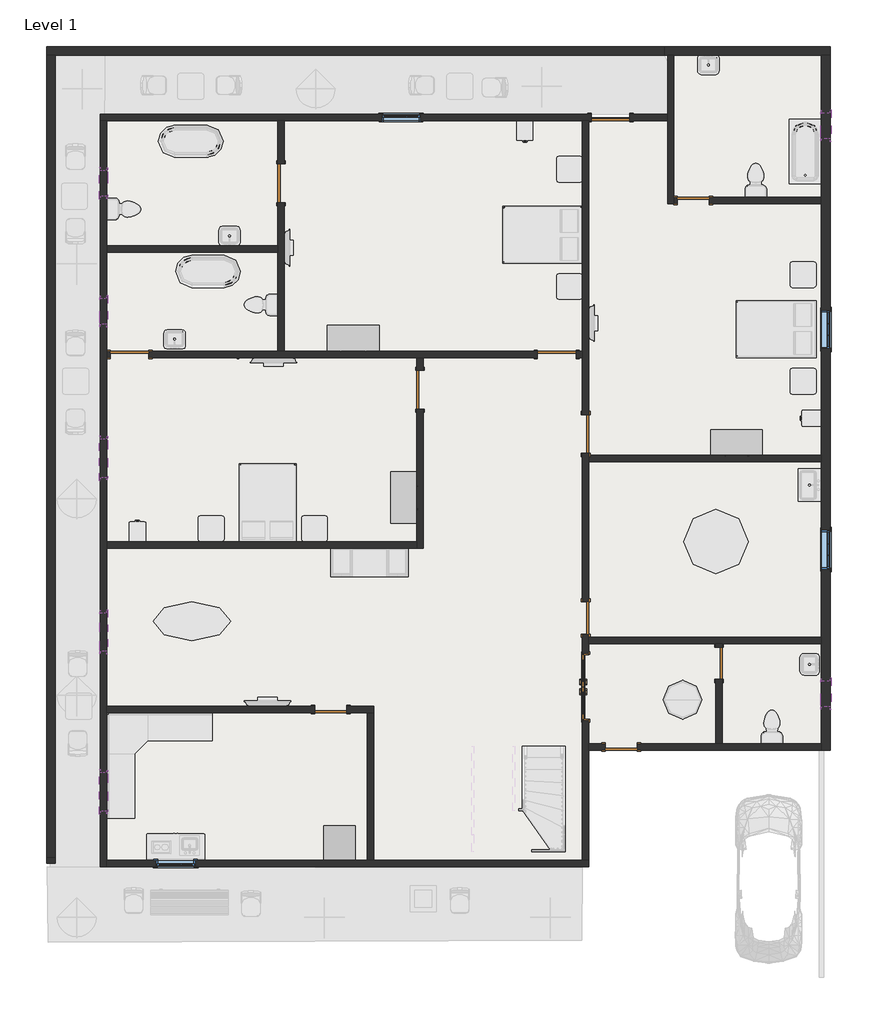
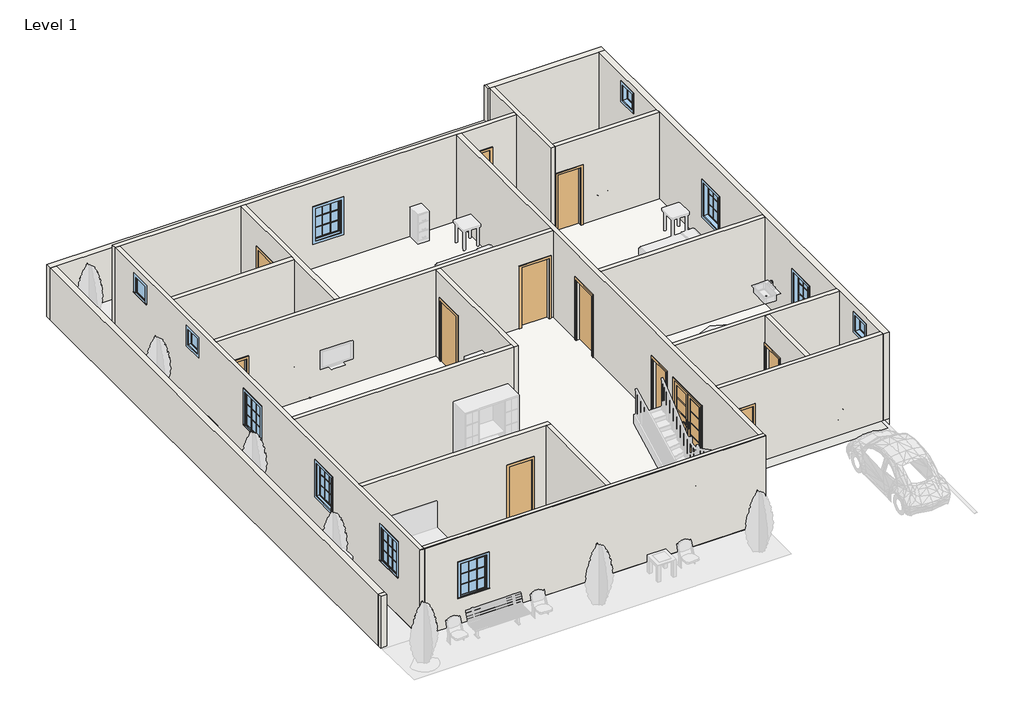
# One storey, part 1 of 3: 22 walls, 12 doors, 11 windows, 1 slab.
"""IFC4 building model written with IfcOpenShell, lengths in millimetres."""

from ifc_helpers import new_model, si_unit, frame, origin, origin_with_axes, place, context, project, spatial, polyline, outline, extrude, faceted_brep, transform, mapped, element, save
from components import door_94998e6c, door_255cab33, door_059fdd7e, door_16372e1c, door_686f89d2, window_5c190c7e, window_29c06734, window_e41d21a6, window_3d781103

model = new_model("IFC4")

# Units and contexts
model_context = context("Model", 3, world=origin())
ifc_project = project(units=[si_unit("LENGTHUNIT", "METRE", prefix="MILLI")], contexts=[model_context])

# Site, building, storey
site = spatial("IfcSite", under=ifc_project)
building = spatial("IfcBuilding", under=site)
storey = spatial("IfcBuildingStorey", under=building, Name="Level 1", Elevation=0.0)

# Doors
placement = place(None, origin())
door_shape = door_94998e6c(model_context)
element("IfcDoor", 1, ObjectType="Door-Exterior-Double-Full Glass-Wood_Clad : 60\" x 80\"", at=placement, inside=storey, context=model_context, shape_type="MappedRepresentation", body=[
    mapped(door_shape, transform((-2733.8668623, -1407.4089531, 0.0), x_axis=(0.0, 1.0, 0.0), y_axis=(-1.0, 0.0, 0.0), z_axis=(0.0, 0.0, 1.0))),
])
door_2_shape = door_255cab33(model_context)
element("IfcDoor", 2, ObjectType="Single-Flush : 30\" x 80\"", at=placement, inside=storey, context=model_context, shape_type="MappedRepresentation", body=[
    mapped(door_2_shape, transform((-190.6918623, 10073.3910469, 0.0), x_axis=(-1.0, 0.0, 0.0), y_axis=(0.0, -1.0, 0.0), z_axis=(0.0, 0.0, 1.0))),
])
element("IfcDoor", 3, ObjectType="Single-Flush : 30\" x 80\"", at=placement, inside=storey, context=model_context, shape_type="MappedRepresentation", body=[
    mapped(door_2_shape, transform((418.9081377, -848.6089531, 0.0), x_axis=(0.0, 1.0, 0.0), y_axis=(-1.0, 0.0, 0.0), z_axis=(0.0, 0.0, 1.0))),
])
element("IfcDoor", 4, ObjectType="Single-Flush : 30\" x 80\"", at=placement, inside=storey, context=model_context, shape_type="MappedRepresentation", body=[
    mapped(door_2_shape, transform((-8750.4918623, -1940.8089531, 0.0), x_axis=(1.0, 0.0, 0.0), y_axis=(0.0, 1.0, 0.0), z_axis=(0.0, 0.0, 1.0))),
])
door_3_shape = door_059fdd7e(model_context)
element("IfcDoor", 5, ObjectType="Single-Flush : 30\" x 80\"", at=placement, inside=storey, context=model_context, shape_type="MappedRepresentation", body=[
    mapped(door_3_shape, transform((-2730.6918623, 218.1910469, 0.0), x_axis=(0.0, -1.0, 0.0), y_axis=(1.0, 0.0, 0.0), z_axis=(0.0, 0.0, 1.0))),
])
element("IfcDoor", 6, ObjectType="Single-Flush : 30\" x 80\"", at=placement, inside=storey, context=model_context, shape_type="MappedRepresentation", body=[
    mapped(door_3_shape, transform((-1892.4918623, -2829.8089531, 0.0), x_axis=(-1.0, 0.0, 0.0), y_axis=(0.0, -1.0, 0.0), z_axis=(0.0, 0.0, 1.0))),
])
door_4_shape = door_16372e1c(model_context)
element("IfcDoor", 7, ObjectType="Single-Flush : 36\" x 84\"", at=placement, inside=storey, context=model_context, shape_type="MappedRepresentation", body=[
    mapped(door_4_shape, transform((-9918.8918623, 10479.7910469, 0.0), x_axis=(0.0, 1.0, 0.0), y_axis=(-1.0, 0.0, 0.0), z_axis=(0.0, 0.0, 1.0))),
])
element("IfcDoor", 8, ObjectType="Single-Flush : 36\" x 84\"", at=placement, inside=storey, context=model_context, shape_type="MappedRepresentation", body=[
    mapped(door_4_shape, transform((-6642.2918623, 5602.9910469, 0.0), x_axis=(0.0, 1.0, 0.0), y_axis=(-1.0, 0.0, 0.0), z_axis=(0.0, 0.0, 1.0))),
])
element("IfcDoor", 9, ObjectType="Single-Flush : 36\" x 84\"", at=placement, inside=storey, context=model_context, shape_type="MappedRepresentation", body=[
    mapped(door_4_shape, transform((-3416.4918623, 6441.1910469, 0.0), x_axis=(1.0, 0.0, 0.0), y_axis=(0.0, 1.0, 0.0), z_axis=(0.0, 0.0, 1.0))),
])
element("IfcDoor", 10, ObjectType="Single-Flush : 36\" x 84\"", at=placement, inside=storey, context=model_context, shape_type="MappedRepresentation", body=[
    mapped(door_4_shape, transform((-2730.6918623, 4561.5910469, 0.0), x_axis=(0.0, -1.0, 0.0), y_axis=(1.0, 0.0, 0.0), z_axis=(0.0, 0.0, 1.0))),
])
element("IfcDoor", 11, ObjectType="Single-Flush : 36\" x 84\"", at=placement, inside=storey, context=model_context, shape_type="MappedRepresentation", body=[
    mapped(door_4_shape, transform((-2146.4918623, 12029.1910469, 0.0), x_axis=(-1.0, 0.0, 0.0), y_axis=(0.0, -1.0, 0.0), z_axis=(0.0, 0.0, 1.0))),
])
door_5_shape = door_686f89d2(model_context)
element("IfcDoor", 12, ObjectType="Single-Flush : 36\" x 84\"", at=placement, inside=storey, context=model_context, shape_type="MappedRepresentation", body=[
    mapped(door_5_shape, transform((-13500.2918623, 6441.1910469, 0.0), x_axis=(-1.0, 0.0, 0.0), y_axis=(0.0, -1.0, 0.0), z_axis=(0.0, 0.0, 1.0))),
])

# Slab
element("IfcSlab", 13, ObjectType="Generic - 12\"", at=placement, inside=storey, context=model_context, shape_type="SweptSolid", body=[
    extrude(outline(polyline([(3035.1081377, -2906.0089531), (-2552.8918623, -2906.0089531), (-2654.4918623, -2906.0089531), (-2654.4918623, -5649.2089531), (-14186.0918623, -5649.2089531), (-14186.0918623, 12029.1910469), (-724.0918623, 12029.1910469), (-724.0918623, 13603.9910469), (3035.1081377, 13603.9910469), (3035.1081377, -2906.0089531)])), frame((0.0, 0.0, -304.8), z_axis=(0.0, 0.0, 1.0), x_axis=(1.0, 0.0, 0.0)), (0.0, 0.0, 1.0), 304.8),
])

# Walls
element("IfcWall", 14, ObjectType="Generic - 8\"", at=placement, inside=storey, context=model_context, shape_type="Brep", body=[
    faceted_brep([(2831.9081377, 13502.3910469, 0.0), (2831.9081377, 10149.5910469, 0.0), (2831.9081377, 9997.1910469, 0.0), (2831.9081377, 4053.5910469, 0.0), (2831.9081377, 3901.1910469, 0.0), (2831.9081377, -239.0089531, 0.0), (2831.9081377, -391.4089531, 0.0), (2831.9081377, -2753.6089531, 0.0), (2831.9081377, -2906.0089531, 0.0), (2831.9081377, -2906.0089531, 3048.0), (2831.9081377, -2753.6089531, 3048.0), (2831.9081377, -391.4089531, 3048.0), (2831.9081377, -239.0089531, 3048.0), (2831.9081377, 3901.1910469, 3048.0), (2831.9081377, 4053.5910469, 3048.0), (2831.9081377, 9997.1910469, 3048.0), (2831.9081377, 10149.5910469, 3048.0), (2831.9081377, 13502.3910469, 3048.0), (2831.9081377, 1373.8910469, 2133.6), (2831.9081377, 1373.8910469, 914.4), (2831.9081377, 2288.2910469, 914.4), (2831.9081377, 2288.2910469, 2133.6), (2831.9081377, 6568.1910469, 2133.6), (2831.9081377, 6568.1910469, 914.4), (2831.9081377, 7482.5910469, 914.4), (2831.9081377, 7482.5910469, 2133.6), (2831.9081377, -1877.3089531, 2768.6), (2831.9081377, -1877.3089531, 2159.0), (2831.9081377, -1267.7089531, 2159.0), (2831.9081377, -1267.7089531, 2768.6), (2831.9081377, 11533.8910469, 2768.6), (2831.9081377, 11533.8910469, 2159.0), (2831.9081377, 12143.4910469, 2159.0), (2831.9081377, 12143.4910469, 2768.6), (3035.1081377, 13502.3910469, 0.0), (3035.1081377, 13502.3910469, 3048.0), (3035.1081377, -2906.0089531, 3048.0), (3035.1081377, -2906.0089531, 0.0), (3035.1081377, 1373.8910469, 2133.6), (3035.1081377, 2288.2910469, 2133.6), (3035.1081377, 2288.2910469, 914.4), (3035.1081377, 1373.8910469, 914.4), (3035.1081377, 6568.1910469, 2133.6), (3035.1081377, 7482.5910469, 2133.6), (3035.1081377, 7482.5910469, 914.4), (3035.1081377, 6568.1910469, 914.4), (3035.1081377, -1877.3089531, 2768.6), (3035.1081377, -1267.7089531, 2768.6), (3035.1081377, -1267.7089531, 2159.0), (3035.1081377, -1877.3089531, 2159.0), (3035.1081377, 11533.8910469, 2768.6), (3035.1081377, 12143.4910469, 2768.6), (3035.1081377, 12143.4910469, 2159.0), (3035.1081377, 11533.8910469, 2159.0)], [[[0, 1, 2, 3, 4, 5, 6, 7, 8, 9, 10, 11, 12, 13, 14, 15, 16, 17], [18, 19, 20, 21], [22, 23, 24, 25], [26, 27, 28, 29], [30, 31, 32, 33]], [[34, 35, 36, 37], [38, 39, 40, 41], [42, 43, 44, 45], [46, 47, 48, 49], [50, 51, 52, 53]], [[8, 7, 6, 5, 4, 3, 2, 1, 0, 34, 37]], [[0, 17, 35, 34]], [[9, 8, 37, 36]], [[19, 18, 38, 41]], [[20, 19, 41, 40]], [[21, 20, 40, 39]], [[18, 21, 39, 38]], [[23, 22, 42, 45]], [[24, 23, 45, 44]], [[25, 24, 44, 43]], [[22, 25, 43, 42]], [[27, 26, 46, 49]], [[28, 27, 49, 48]], [[29, 28, 48, 47]], [[26, 29, 47, 46]], [[31, 30, 50, 53]], [[32, 31, 53, 52]], [[33, 32, 52, 51]], [[30, 33, 51, 50]], [[17, 16, 15, 14, 13, 12, 11, 10, 9, 36, 35]]]),
])
element("IfcWall", 15, ObjectType="Generic - 8\"", at=placement, inside=storey, context=model_context, shape_type="SweptSolid", body=[
    extrude(outline(polyline([(-15252.8918623, -5446.0089531), (-15252.8918623, -5573.0089531), (-15456.0918623, -5573.0089531), (-15456.0918623, -5446.0089531), (-15252.8918623, -5446.0089531)])), origin_with_axes(), (0.0, 0.0, 1.0), 1828.8),
])
element("IfcWall", 16, ObjectType="Generic - 8\"", at=placement, inside=storey, context=model_context, shape_type="Brep", body=[
    faceted_brep([(-876.4918623, 13502.3910469, 0.0), (-800.2918623, 13502.3910469, 0.0), (-647.8918623, 13502.3910469, 0.0), (2831.9081377, 13502.3910469, 0.0), (3035.1081377, 13502.3910469, 0.0), (3035.1081377, 13502.3910469, 3048.0), (2831.9081377, 13502.3910469, 3048.0), (-647.8918623, 13502.3910469, 3048.0), (-800.2918623, 13502.3910469, 3048.0), (-876.4918623, 13502.3910469, 3048.0), (-876.4918623, 13705.5910469, 0.0), (-876.4918623, 13705.5910469, 3048.0), (-800.2918623, 13705.5910469, 3048.0), (3035.1081377, 13705.5910469, 3048.0), (3035.1081377, 13705.5910469, 0.0)], [[[0, 1, 2, 3, 4, 5, 6, 7, 8, 9]], [[10, 11, 12, 13, 14]], [[4, 3, 2, 1, 0, 10, 14]], [[0, 9, 11, 10]], [[5, 4, 14, 13]], [[9, 8, 12, 11]], [[8, 7, 6, 5, 13, 12]]]),
])
element("IfcWall", 17, ObjectType="Generic - 8\" 2", at=placement, inside=storey, context=model_context, shape_type="Brep", body=[
    faceted_brep([(-15456.0918623, 13502.3910469, 0.0), (-15252.8918623, 13502.3910469, 0.0), (-876.4918623, 13502.3910469, 0.0), (-876.4918623, 13502.3910469, 1828.8), (-15252.8918623, 13502.3910469, 1828.8), (-15456.0918623, 13502.3910469, 1828.8), (-15456.0918623, 13705.5910469, 0.0), (-15456.0918623, 13705.5910469, 1828.8), (-876.4918623, 13705.5910469, 1828.8), (-876.4918623, 13705.5910469, 0.0)], [[[0, 1, 2, 3, 4, 5]], [[6, 7, 8, 9]], [[2, 1, 0, 6, 9]], [[3, 2, 9, 8]], [[5, 4, 3, 8, 7]], [[0, 5, 7, 6]]]),
])
element("IfcWall", 18, ObjectType="Generic - 8\" 2", at=placement, inside=storey, context=model_context, shape_type="SweptSolid", body=[
    extrude(outline(polyline([(-15252.8918623, 13502.3910469), (-15252.8918623, -5446.0089531), (-15456.0918623, -5446.0089531), (-15456.0918623, 13502.3910469), (-15252.8918623, 13502.3910469)])), origin_with_axes(), (0.0, 0.0, 1.0), 1828.8),
])
element("IfcWall", 19, ObjectType="INNER WALL", at=placement, inside=storey, context=model_context, shape_type="Brep", body=[
    faceted_brep([(-800.2918623, 13502.3910469, 0.0), (-800.2918623, 12105.3910469, 0.0), (-800.2918623, 11952.9910469, 0.0), (-800.2918623, 9997.1910469, 0.0), (-800.2918623, 9997.1910469, 3048.0), (-800.2918623, 11952.9910469, 3048.0), (-800.2918623, 12105.3910469, 3048.0), (-800.2918623, 13502.3910469, 3048.0), (-647.8918623, 13502.3910469, 0.0), (-647.8918623, 13502.3910469, 3048.0), (-647.8918623, 10149.5910469, 3048.0), (-647.8918623, 9997.1910469, 3048.0), (-647.8918623, 9997.1910469, 0.0), (-647.8918623, 10149.5910469, 0.0)], [[[0, 1, 2, 3, 4, 5, 6, 7]], [[8, 9, 10, 11, 12, 13]], [[3, 2, 1, 0, 8, 13, 12]], [[0, 7, 9, 8]], [[4, 3, 12, 11]], [[7, 6, 5, 4, 11, 10, 9]]]),
])
element("IfcWall", 20, ObjectType="INNER WALL", at=placement, inside=storey, context=model_context, shape_type="SweptSolid", body=[
    extrude(outline(polyline([(0.0, -647.8918623), (0.0, -571.6918623), (2032.0, -571.6918623), (2032.0, 190.3081377), (0.0, 190.3081377), (0.0, 2831.9081377), (3048.0, 2831.9081377), (3048.0, -647.8918623), (0.0, -647.8918623)])), frame((0.0, 9997.1910469, 0.0), z_axis=(0.0, 1.0, 0.0), x_axis=(0.0, 0.0, 1.0)), (0.0, 0.0, 1.0), 152.4),
])
element("IfcWall", 21, ObjectType="INNER WALL", at=placement, inside=storey, context=model_context, shape_type="Brep", body=[
    faceted_brep([(-2603.6918623, 12105.3910469, 2133.6), (-2603.6918623, 12105.3910469, 0.0), (-14186.0918623, 12105.3910469, 0.0), (-14186.0918623, 12105.3910469, 3048.0), (-800.2918623, 12105.3910469, 3048.0), (-800.2918623, 12105.3910469, 0.0), (-1689.2918623, 12105.3910469, 0.0), (-1689.2918623, 12105.3910469, 2133.6), (-6629.5918623, 12105.3910469, 2133.6), (-7543.9918623, 12105.3910469, 2133.6), (-7543.9918623, 12105.3910469, 914.4), (-6629.5918623, 12105.3910469, 914.4), (-14186.0918623, 11952.9910469, 0.0), (-14033.6918623, 11952.9910469, 0.0), (-9995.0918623, 11952.9910469, 0.0), (-9842.6918623, 11952.9910469, 0.0), (-2806.8918623, 11952.9910469, 0.0), (-2654.4918623, 11952.9910469, 0.0), (-2603.6918623, 11952.9910469, 0.0), (-2603.6918623, 11952.9910469, 2133.6), (-1689.2918623, 11952.9910469, 2133.6), (-1689.2918623, 11952.9910469, 0.0), (-800.2918623, 11952.9910469, 0.0), (-800.2918623, 11952.9910469, 3048.0), (-2654.4918623, 11952.9910469, 3048.0), (-2806.8918623, 11952.9910469, 3048.0), (-9842.6918623, 11952.9910469, 3048.0), (-9995.0918623, 11952.9910469, 3048.0), (-14033.6918623, 11952.9910469, 3048.0), (-14186.0918623, 11952.9910469, 3048.0), (-6629.5918623, 11952.9910469, 2133.6), (-6629.5918623, 11952.9910469, 914.4), (-7543.9918623, 11952.9910469, 914.4), (-7543.9918623, 11952.9910469, 2133.6)], [[[0, 1, 2, 3, 4, 5, 6, 7], [8, 9, 10, 11]], [[12, 13, 14, 15, 16, 17, 18, 19, 20, 21, 22, 23, 24, 25, 26, 27, 28, 29], [30, 31, 32, 33]], [[6, 5, 22, 21]], [[2, 1, 18, 17, 16, 15, 14, 13, 12]], [[5, 4, 23, 22]], [[3, 2, 12, 29]], [[19, 18, 1, 0]], [[20, 19, 0, 7]], [[21, 20, 7, 6]], [[31, 30, 8, 11]], [[32, 31, 11, 10]], [[33, 32, 10, 9]], [[30, 33, 9, 8]], [[4, 3, 29, 28, 27, 26, 25, 24, 23]]]),
])
element("IfcWall", 22, ObjectType="INNER WALL", at=placement, inside=storey, context=model_context, shape_type="Brep", body=[
    faceted_brep([(-2806.8918623, 11952.9910469, 3048.0), (-2806.8918623, 11952.9910469, 0.0), (-2806.8918623, 6517.3910469, 0.0), (-2806.8918623, 6364.9910469, 0.0), (-2806.8918623, 5018.7910469, 0.0), (-2806.8918623, 5018.7910469, 2133.6), (-2806.8918623, 4104.3910469, 2133.6), (-2806.8918623, 4104.3910469, 0.0), (-2806.8918623, 599.1910469, 0.0), (-2806.8918623, 599.1910469, 2032.0), (-2806.8918623, -162.8089531, 2032.0), (-2806.8918623, -162.8089531, 0.0), (-2806.8918623, -620.0089531, 0.0), (-2806.8918623, -620.0089531, 2057.4), (-2806.8918623, -2194.8089531, 2057.4), (-2806.8918623, -2194.8089531, 0.0), (-2806.8918623, -5496.8089531, 0.0), (-2806.8918623, -5496.8089531, 3048.0), (-2806.8918623, 6364.9910469, 3048.0), (-2806.8918623, 6517.3910469, 3048.0), (-2654.4918623, 11952.9910469, 0.0), (-2654.4918623, 11952.9910469, 3048.0), (-2654.4918623, 4053.5910469, 3048.0), (-2654.4918623, 3901.1910469, 3048.0), (-2654.4918623, -239.0089531, 3048.0), (-2654.4918623, -391.4089531, 3048.0), (-2654.4918623, -2753.6089531, 3048.0), (-2654.4918623, -2906.0089531, 3048.0), (-2654.4918623, -5496.8089531, 3048.0), (-2654.4918623, -5496.8089531, 0.0), (-2654.4918623, -2906.0089531, 0.0), (-2654.4918623, -2753.6089531, 0.0), (-2654.4918623, -2194.8089531, 0.0), (-2654.4918623, -2194.8089531, 2057.4), (-2654.4918623, -620.0089531, 2057.4), (-2654.4918623, -620.0089531, 0.0), (-2654.4918623, -391.4089531, 0.0), (-2654.4918623, -239.0089531, 0.0), (-2654.4918623, -162.8089531, 0.0), (-2654.4918623, -162.8089531, 2032.0), (-2654.4918623, 599.1910469, 2032.0), (-2654.4918623, 599.1910469, 0.0), (-2654.4918623, 3901.1910469, 0.0), (-2654.4918623, 4053.5910469, 0.0), (-2654.4918623, 4104.3910469, 0.0), (-2654.4918623, 4104.3910469, 2133.6), (-2654.4918623, 5018.7910469, 2133.6), (-2654.4918623, 5018.7910469, 0.0)], [[[0, 1, 2, 3, 4, 5, 6, 7, 8, 9, 10, 11, 12, 13, 14, 15, 16, 17, 18, 19]], [[20, 21, 22, 23, 24, 25, 26, 27, 28, 29, 30, 31, 32, 33, 34, 35, 36, 37, 38, 39, 40, 41, 42, 43, 44, 45, 46, 47]], [[1, 20, 47, 4, 3, 2]], [[7, 44, 43, 42, 41, 8]], [[11, 38, 37, 36, 35, 12]], [[29, 16, 15, 32, 31, 30]], [[1, 0, 21, 20]], [[45, 44, 7, 6]], [[46, 45, 6, 5]], [[47, 46, 5, 4]], [[39, 38, 11, 10]], [[40, 39, 10, 9]], [[41, 40, 9, 8]], [[34, 13, 12, 35]], [[13, 34, 33, 14]], [[14, 33, 32, 15]], [[17, 16, 29, 28]], [[21, 0, 19, 18, 17, 28, 27, 26, 25, 24, 23, 22]]]),
])
element("IfcWall", 23, ObjectType="INNER WALL", at=placement, inside=storey, context=model_context, shape_type="SweptSolid", body=[
    extrude(outline(polyline([(2831.9081377, 3901.1910469), (-2654.4918623, 3901.1910469), (-2654.4918623, 4053.5910469), (2831.9081377, 4053.5910469), (2831.9081377, 3901.1910469)])), origin_with_axes(), (0.0, 0.0, 1.0), 3048.0),
])
element("IfcWall", 24, ObjectType="INNER WALL", at=placement, inside=storey, context=model_context, shape_type="Brep", body=[
    faceted_brep([(-2654.4918623, -391.4089531, 0.0), (342.7081377, -391.4089531, 0.0), (495.1081377, -391.4089531, 0.0), (2831.9081377, -391.4089531, 0.0), (2831.9081377, -391.4089531, 3048.0), (495.1081377, -391.4089531, 3048.0), (342.7081377, -391.4089531, 3048.0), (-2654.4918623, -391.4089531, 3048.0), (-2654.4918623, -239.0089531, 0.0), (-2654.4918623, -239.0089531, 3048.0), (2831.9081377, -239.0089531, 3048.0), (2831.9081377, -239.0089531, 0.0)], [[[0, 1, 2, 3, 4, 5, 6, 7]], [[8, 9, 10, 11]], [[3, 2, 1, 0, 8, 11]], [[0, 7, 9, 8]], [[4, 3, 11, 10]], [[7, 6, 5, 4, 10, 9]]]),
])
element("IfcWall", 25, ObjectType="INNER WALL", at=placement, inside=storey, context=model_context, shape_type="Brep", body=[
    faceted_brep([(-2273.4918623, -2753.6089531, 2032.0), (-2273.4918623, -2753.6089531, 0.0), (-2654.4918623, -2753.6089531, 0.0), (-2654.4918623, -2753.6089531, 3048.0), (342.7081377, -2753.6089531, 3048.0), (495.1081377, -2753.6089531, 3048.0), (2831.9081377, -2753.6089531, 3048.0), (2831.9081377, -2753.6089531, 0.0), (495.1081377, -2753.6089531, 0.0), (342.7081377, -2753.6089531, 0.0), (-1511.4918623, -2753.6089531, 0.0), (-1511.4918623, -2753.6089531, 2032.0), (-2654.4918623, -2906.0089531, 0.0), (-2273.4918623, -2906.0089531, 0.0), (-2273.4918623, -2906.0089531, 2032.0), (-1511.4918623, -2906.0089531, 2032.0), (-1511.4918623, -2906.0089531, 0.0), (2831.9081377, -2906.0089531, 0.0), (2831.9081377, -2906.0089531, 3048.0), (-2654.4918623, -2906.0089531, 3048.0)], [[[0, 1, 2, 3, 4, 5, 6, 7, 8, 9, 10, 11]], [[12, 13, 14, 15, 16, 17, 18, 19]], [[2, 1, 13, 12]], [[10, 9, 8, 7, 17, 16]], [[7, 6, 18, 17]], [[3, 2, 12, 19]], [[14, 13, 1, 0]], [[15, 14, 0, 11]], [[16, 15, 11, 10]], [[6, 5, 4, 3, 19, 18]]]),
])
element("IfcWall", 26, ObjectType="INNER WALL", at=placement, inside=storey, context=model_context, shape_type="Brep", body=[
    faceted_brep([(-14186.0918623, 11952.9910469, 0.0), (-14186.0918623, -5649.2089531, 0.0), (-14186.0918623, -5649.2089531, 3048.0), (-14186.0918623, -5623.8089531, 3048.0), (-14186.0918623, 11952.9910469, 3048.0), (-14186.0918623, 4447.2910469, 2540.0), (-14186.0918623, 3532.8910469, 2540.0), (-14186.0918623, 3532.8910469, 1320.8), (-14186.0918623, 4447.2910469, 1320.8), (-14186.0918623, -569.2089531, 2540.0), (-14186.0918623, -569.2089531, 1320.8), (-14186.0918623, 345.1910469, 1320.8), (-14186.0918623, 345.1910469, 2540.0), (-14186.0918623, -3426.7089531, 2540.0), (-14186.0918623, -4341.1089531, 2540.0), (-14186.0918623, -4341.1089531, 1320.8), (-14186.0918623, -3426.7089531, 1320.8), (-14186.0918623, 10784.5910469, 2768.6), (-14186.0918623, 10174.9910469, 2768.6), (-14186.0918623, 10174.9910469, 2159.0), (-14186.0918623, 10784.5910469, 2159.0), (-14186.0918623, 7152.3910469, 2768.6), (-14186.0918623, 7152.3910469, 2159.0), (-14186.0918623, 7761.9910469, 2159.0), (-14186.0918623, 7761.9910469, 2768.6), (-14033.6918623, 11952.9910469, 0.0), (-14033.6918623, 11952.9910469, 3048.0), (-14033.6918623, 9006.5910469, 3048.0), (-14033.6918623, 8854.1910469, 3048.0), (-14033.6918623, 6517.3910469, 3048.0), (-14033.6918623, 6364.9910469, 3048.0), (-14033.6918623, 2021.5910469, 3048.0), (-14033.6918623, 1869.1910469, 3048.0), (-14033.6918623, -1864.6089531, 3048.0), (-14033.6918623, -2017.0089531, 3048.0), (-14033.6918623, -5496.8089531, 3048.0), (-14033.6918623, -5623.8089531, 3048.0), (-14033.6918623, -5649.2089531, 3048.0), (-14033.6918623, -5649.2089531, 0.0), (-14033.6918623, -5496.8089531, 0.0), (-14033.6918623, -2017.0089531, 0.0), (-14033.6918623, -1864.6089531, 0.0), (-14033.6918623, 1869.1910469, 0.0), (-14033.6918623, 2021.5910469, 0.0), (-14033.6918623, 6364.9910469, 0.0), (-14033.6918623, 6517.3910469, 0.0), (-14033.6918623, 8854.1910469, 0.0), (-14033.6918623, 9006.5910469, 0.0), (-14033.6918623, 4447.2910469, 2540.0), (-14033.6918623, 4447.2910469, 1320.8), (-14033.6918623, 3532.8910469, 1320.8), (-14033.6918623, 3532.8910469, 2540.0), (-14033.6918623, -569.2089531, 2540.0), (-14033.6918623, 345.1910469, 2540.0), (-14033.6918623, 345.1910469, 1320.8), (-14033.6918623, -569.2089531, 1320.8), (-14033.6918623, -3426.7089531, 2540.0), (-14033.6918623, -3426.7089531, 1320.8), (-14033.6918623, -4341.1089531, 1320.8), (-14033.6918623, -4341.1089531, 2540.0), (-14033.6918623, 10784.5910469, 2768.6), (-14033.6918623, 10784.5910469, 2159.0), (-14033.6918623, 10174.9910469, 2159.0), (-14033.6918623, 10174.9910469, 2768.6), (-14033.6918623, 7152.3910469, 2768.6), (-14033.6918623, 7761.9910469, 2768.6), (-14033.6918623, 7761.9910469, 2159.0), (-14033.6918623, 7152.3910469, 2159.0)], [[[0, 1, 2, 3, 4], [5, 6, 7, 8], [9, 10, 11, 12], [13, 14, 15, 16], [17, 18, 19, 20], [21, 22, 23, 24]], [[25, 26, 27, 28, 29, 30, 31, 32, 33, 34, 35, 36, 37, 38, 39, 40, 41, 42, 43, 44, 45, 46, 47], [48, 49, 50, 51], [52, 53, 54, 55], [56, 57, 58, 59], [60, 61, 62, 63], [64, 65, 66, 67]], [[1, 0, 25, 47, 46, 45, 44, 43, 42, 41, 40, 39, 38]], [[0, 4, 26, 25]], [[49, 48, 5, 8]], [[50, 49, 8, 7]], [[51, 50, 7, 6]], [[48, 51, 6, 5]], [[10, 9, 52, 55]], [[11, 10, 55, 54]], [[12, 11, 54, 53]], [[9, 12, 53, 52]], [[57, 56, 13, 16]], [[58, 57, 16, 15]], [[59, 58, 15, 14]], [[56, 59, 14, 13]], [[61, 60, 17, 20]], [[62, 61, 20, 19]], [[63, 62, 19, 18]], [[60, 63, 18, 17]], [[22, 21, 64, 67]], [[23, 22, 67, 66]], [[24, 23, 66, 65]], [[21, 24, 65, 64]], [[2, 1, 38, 37]], [[3, 2, 37, 36]], [[4, 3, 36, 35, 34, 33, 32, 31, 30, 29, 28, 27, 26]]]),
])
element("IfcWall", 27, ObjectType="INNER WALL", at=placement, inside=storey, context=model_context, shape_type="Brep", body=[
    faceted_brep([(-2959.2918623, 6364.9910469, 2133.6), (-2959.2918623, 6364.9910469, 0.0), (-2806.8918623, 6364.9910469, 0.0), (-2806.8918623, 6364.9910469, 3048.0), (-6566.0918623, 6364.9910469, 3048.0), (-6718.4918623, 6364.9910469, 3048.0), (-14033.6918623, 6364.9910469, 3048.0), (-14033.6918623, 6364.9910469, 0.0), (-13957.4918623, 6364.9910469, 0.0), (-13957.4918623, 6364.9910469, 2133.6), (-13043.0918623, 6364.9910469, 2133.6), (-13043.0918623, 6364.9910469, 0.0), (-6718.4918623, 6364.9910469, 0.0), (-6566.0918623, 6364.9910469, 0.0), (-3873.6918623, 6364.9910469, 0.0), (-3873.6918623, 6364.9910469, 2133.6), (-2806.8918623, 6517.3910469, 0.0), (-2959.2918623, 6517.3910469, 0.0), (-2959.2918623, 6517.3910469, 2133.6), (-3873.6918623, 6517.3910469, 2133.6), (-3873.6918623, 6517.3910469, 0.0), (-9842.6918623, 6517.3910469, 0.0), (-9995.0918623, 6517.3910469, 0.0), (-13043.0918623, 6517.3910469, 0.0), (-13043.0918623, 6517.3910469, 2133.6), (-13957.4918623, 6517.3910469, 2133.6), (-13957.4918623, 6517.3910469, 0.0), (-14033.6918623, 6517.3910469, 0.0), (-14033.6918623, 6517.3910469, 3048.0), (-9995.0918623, 6517.3910469, 3048.0), (-9842.6918623, 6517.3910469, 3048.0), (-2806.8918623, 6517.3910469, 3048.0)], [[[0, 1, 2, 3, 4, 5, 6, 7, 8, 9, 10, 11, 12, 13, 14, 15]], [[16, 17, 18, 19, 20, 21, 22, 23, 24, 25, 26, 27, 28, 29, 30, 31]], [[27, 26, 8, 7]], [[2, 1, 17, 16]], [[14, 13, 12, 11, 23, 22, 21, 20]], [[3, 2, 16, 31]], [[7, 6, 28, 27]], [[9, 8, 26, 25]], [[10, 9, 25, 24]], [[11, 10, 24, 23]], [[18, 17, 1, 0]], [[19, 18, 0, 15]], [[20, 19, 15, 14]], [[6, 5, 4, 3, 31, 30, 29, 28]]]),
])
element("IfcWall", 28, ObjectType="INNER WALL", at=placement, inside=storey, context=model_context, shape_type="Brep", body=[
    faceted_brep([(-6718.4918623, 6364.9910469, 0.0), (-6718.4918623, 6060.1910469, 0.0), (-6718.4918623, 6060.1910469, 2133.6), (-6718.4918623, 5145.7910469, 2133.6), (-6718.4918623, 5145.7910469, 0.0), (-6718.4918623, 2021.5910469, 0.0), (-6718.4918623, 1869.1910469, 0.0), (-6718.4918623, 1869.1910469, 3048.0), (-6718.4918623, 2021.5910469, 3048.0), (-6718.4918623, 6364.9910469, 3048.0), (-6566.0918623, 6060.1910469, 2133.6), (-6566.0918623, 6060.1910469, 0.0), (-6566.0918623, 6364.9910469, 0.0), (-6566.0918623, 6364.9910469, 3048.0), (-6566.0918623, 1869.1910469, 3048.0), (-6566.0918623, 1869.1910469, 0.0), (-6566.0918623, 5145.7910469, 0.0), (-6566.0918623, 5145.7910469, 2133.6)], [[[0, 1, 2, 3, 4, 5, 6, 7, 8, 9]], [[10, 11, 12, 13, 14, 15, 16, 17]], [[16, 15, 6, 5, 4]], [[12, 11, 1, 0]], [[0, 9, 13, 12]], [[7, 6, 15, 14]], [[2, 1, 11, 10]], [[3, 2, 10, 17]], [[4, 3, 17, 16]], [[9, 8, 7, 14, 13]]]),
])
element("IfcWall", 29, ObjectType="INNER WALL", at=placement, inside=storey, context=model_context, shape_type="SweptSolid", body=[
    extrude(outline(polyline([(-14033.6918623, 2021.5910469), (-6718.4918623, 2021.5910469), (-6718.4918623, 1869.1910469), (-14033.6918623, 1869.1910469), (-14033.6918623, 2021.5910469)])), origin_with_axes(), (0.0, 0.0, 1.0), 3048.0),
])
element("IfcWall", 30, ObjectType="INNER WALL", at=placement, inside=storey, context=model_context, shape_type="Brep", body=[
    faceted_brep([(-9995.0918623, 11952.9910469, 0.0), (-9995.0918623, 10936.9910469, 0.0), (-9995.0918623, 10936.9910469, 2133.6), (-9995.0918623, 10022.5910469, 2133.6), (-9995.0918623, 10022.5910469, 0.0), (-9995.0918623, 9006.5910469, 0.0), (-9995.0918623, 8854.1910469, 0.0), (-9995.0918623, 6517.3910469, 0.0), (-9995.0918623, 6517.3910469, 3048.0), (-9995.0918623, 8854.1910469, 3048.0), (-9995.0918623, 9006.5910469, 3048.0), (-9995.0918623, 11952.9910469, 3048.0), (-9842.6918623, 10936.9910469, 2133.6), (-9842.6918623, 10936.9910469, 0.0), (-9842.6918623, 11952.9910469, 0.0), (-9842.6918623, 11952.9910469, 3048.0), (-9842.6918623, 6517.3910469, 3048.0), (-9842.6918623, 6517.3910469, 0.0), (-9842.6918623, 10022.5910469, 0.0), (-9842.6918623, 10022.5910469, 2133.6)], [[[0, 1, 2, 3, 4, 5, 6, 7, 8, 9, 10, 11]], [[12, 13, 14, 15, 16, 17, 18, 19]], [[18, 17, 7, 6, 5, 4]], [[14, 13, 1, 0]], [[0, 11, 15, 14]], [[8, 7, 17, 16]], [[2, 1, 13, 12]], [[3, 2, 12, 19]], [[4, 3, 19, 18]], [[11, 10, 9, 8, 16, 15]]]),
])
element("IfcWall", 31, ObjectType="INNER WALL", at=placement, inside=storey, context=model_context, shape_type="SweptSolid", body=[
    extrude(outline(polyline([(-9995.0918623, 8854.1910469), (-14033.6918623, 8854.1910469), (-14033.6918623, 9006.5910469), (-9995.0918623, 9006.5910469), (-9995.0918623, 8854.1910469)])), origin_with_axes(), (0.0, 0.0, 1.0), 3048.0),
])
element("IfcWall", 32, ObjectType="INNER WALL", at=placement, inside=storey, context=model_context, shape_type="SweptSolid", body=[
    extrude(outline(polyline([(-391.4089531, 0.0), (-467.6089531, 0.0), (-467.6089531, 2032.0), (-1229.6089531, 2032.0), (-1229.6089531, 0.0), (-2753.6089531, 0.0), (-2753.6089531, 3048.0), (-391.4089531, 3048.0), (-391.4089531, 0.0)])), frame((342.7081377, 0.0, 0.0), z_axis=(1.0, 0.0, 0.0), x_axis=(0.0, 1.0, 0.0)), (0.0, 0.0, 1.0), 152.4),
])
element("IfcWall", 33, ObjectType="INNER WALL", at=placement, inside=storey, context=model_context, shape_type="Brep", body=[
    faceted_brep([(-8369.4918623, -2017.0089531, 2032.0), (-8369.4918623, -2017.0089531, 0.0), (-7886.8918623, -2017.0089531, 0.0), (-7734.4918623, -2017.0089531, 0.0), (-7734.4918623, -2017.0089531, 3048.0), (-7886.8918623, -2017.0089531, 3048.0), (-14033.6918623, -2017.0089531, 3048.0), (-14033.6918623, -2017.0089531, 0.0), (-9131.4918623, -2017.0089531, 0.0), (-9131.4918623, -2017.0089531, 2032.0), (-7734.4918623, -1864.6089531, 0.0), (-8369.4918623, -1864.6089531, 0.0), (-8369.4918623, -1864.6089531, 2032.0), (-9131.4918623, -1864.6089531, 2032.0), (-9131.4918623, -1864.6089531, 0.0), (-14033.6918623, -1864.6089531, 0.0), (-14033.6918623, -1864.6089531, 3048.0), (-7734.4918623, -1864.6089531, 3048.0)], [[[0, 1, 2, 3, 4, 5, 6, 7, 8, 9]], [[10, 11, 12, 13, 14, 15, 16, 17]], [[8, 7, 15, 14]], [[3, 2, 1, 11, 10]], [[7, 6, 16, 15]], [[12, 11, 1, 0]], [[13, 12, 0, 9]], [[14, 13, 9, 8]], [[4, 3, 10, 17]], [[6, 5, 4, 17, 16]]]),
])
element("IfcWall", 34, ObjectType="INNER WALL", at=placement, inside=storey, context=model_context, shape_type="SweptSolid", body=[
    extrude(outline(polyline([(-7886.8918623, -5496.8089531), (-7886.8918623, -2017.0089531), (-7734.4918623, -2017.0089531), (-7734.4918623, -5496.8089531), (-7886.8918623, -5496.8089531)])), origin_with_axes(), (0.0, 0.0, 1.0), 3048.0),
])
element("IfcWall", 35, ObjectType="INNER WALL", at=placement, inside=storey, context=model_context, shape_type="Brep", body=[
    faceted_brep([(-2654.4918623, -5496.8089531, 0.0), (-2806.8918623, -5496.8089531, 0.0), (-7734.4918623, -5496.8089531, 0.0), (-7886.8918623, -5496.8089531, 0.0), (-14033.6918623, -5496.8089531, 0.0), (-14033.6918623, -5496.8089531, 3048.0), (-7886.8918623, -5496.8089531, 3048.0), (-7734.4918623, -5496.8089531, 3048.0), (-2806.8918623, -5496.8089531, 3048.0), (-2654.4918623, -5496.8089531, 3048.0), (-12865.2918623, -5496.8089531, 2133.6), (-12865.2918623, -5496.8089531, 914.4), (-11950.8918623, -5496.8089531, 914.4), (-11950.8918623, -5496.8089531, 2133.6), (-2654.4918623, -5649.2089531, 0.0), (-2654.4918623, -5649.2089531, 3048.0), (-14033.6918623, -5649.2089531, 3048.0), (-14033.6918623, -5649.2089531, 0.0), (-12865.2918623, -5649.2089531, 2133.6), (-11950.8918623, -5649.2089531, 2133.6), (-11950.8918623, -5649.2089531, 914.4), (-12865.2918623, -5649.2089531, 914.4), (-2654.4918623, -5623.8089531, 3048.0), (-14033.6918623, -5623.8089531, 3048.0)], [[[0, 1, 2, 3, 4, 5, 6, 7, 8, 9], [10, 11, 12, 13]], [[14, 15, 16, 17], [18, 19, 20, 21]], [[4, 3, 2, 1, 0, 14, 17]], [[10, 13, 19, 18]], [[13, 12, 20, 19]], [[12, 11, 21, 20]], [[11, 10, 18, 21]], [[0, 9, 22, 15, 14]], [[5, 4, 17, 16, 23]], [[23, 16, 15, 22]], [[9, 8, 7, 6, 5, 23, 22]]]),
])

# Windows
window_shape = window_5c190c7e(model_context)
element("IfcWindow", 36, ObjectType="Casement 3x3 with Trim : 36\" x 48\"", at=placement, inside=storey, context=model_context, shape_type="MappedRepresentation", body=[
    mapped(window_shape, transform((-7086.7918623, 12029.1910469, 0.0), x_axis=(1.0, 0.0, 0.0), y_axis=(0.0, 1.0, 0.0), z_axis=(0.0, 0.0, 1.0))),
])
element("IfcWindow", 37, ObjectType="Casement 3x3 with Trim : 36\" x 48\"", at=placement, inside=storey, context=model_context, shape_type="MappedRepresentation", body=[
    mapped(window_shape, transform((-14109.8918623, 3990.0910469, 406.4), x_axis=(0.0, 1.0, 0.0), y_axis=(-1.0, 0.0, 0.0), z_axis=(0.0, 0.0, 1.0))),
])
element("IfcWindow", 38, ObjectType="Casement 3x3 with Trim : 36\" x 48\"", at=placement, inside=storey, context=model_context, shape_type="MappedRepresentation", body=[
    mapped(window_shape, transform((-14109.8918623, -112.0089531, 406.4), x_axis=(0.0, -1.0, 0.0), y_axis=(1.0, 0.0, 0.0), z_axis=(0.0, 0.0, 1.0))),
])
element("IfcWindow", 39, ObjectType="Casement 3x3 with Trim : 36\" x 48\"", at=placement, inside=storey, context=model_context, shape_type="MappedRepresentation", body=[
    mapped(window_shape, transform((-14109.8918623, -3883.9089531, 406.4), x_axis=(0.0, 1.0, 0.0), y_axis=(-1.0, 0.0, 0.0), z_axis=(0.0, 0.0, 1.0))),
])
element("IfcWindow", 40, ObjectType="Casement 3x3 with Trim : 36\" x 48\"", at=placement, inside=storey, context=model_context, shape_type="MappedRepresentation", body=[
    mapped(window_shape, transform((-12408.0918623, -5573.0089531, 0.0), x_axis=(-1.0, 0.0, 0.0), y_axis=(0.0, -1.0, 0.0), z_axis=(0.0, 0.0, 1.0))),
])
window_2_shape = window_29c06734(model_context)
element("IfcWindow", 41, ObjectType="Casement 3x3 with Trim : 36\" x 48\"", at=placement, inside=storey, context=model_context, shape_type="MappedRepresentation", body=[
    mapped(window_2_shape, transform((2933.5081377, 1831.0910469, 0.0), x_axis=(0.0, -1.0, 0.0), y_axis=(1.0, 0.0, 0.0), z_axis=(0.0, 0.0, 1.0))),
])
element("IfcWindow", 42, ObjectType="Casement 3x3 with Trim : 36\" x 48\"", at=placement, inside=storey, context=model_context, shape_type="MappedRepresentation", body=[
    mapped(window_2_shape, transform((2933.5081377, 7025.3910469, 0.0), x_axis=(0.0, -1.0, 0.0), y_axis=(1.0, 0.0, 0.0), z_axis=(0.0, 0.0, 1.0))),
])
window_3_shape = window_e41d21a6(model_context)
element("IfcWindow", 43, ObjectType="Transom with Trim : 24\" x 24\"", at=placement, inside=storey, context=model_context, shape_type="MappedRepresentation", body=[
    mapped(window_3_shape, transform((2933.5081377, -1610.6089531, 0.0), x_axis=(0.0, -1.0, 0.0), y_axis=(1.0, 0.0, 0.0), z_axis=(0.0, 0.0, 1.0))),
])
element("IfcWindow", 44, ObjectType="Transom with Trim : 24\" x 24\"", at=placement, inside=storey, context=model_context, shape_type="MappedRepresentation", body=[
    mapped(window_3_shape, transform((2933.5081377, 11800.5910469, 0.0), x_axis=(0.0, -1.0, 0.0), y_axis=(1.0, 0.0, 0.0), z_axis=(0.0, 0.0, 1.0))),
])
window_4_shape = window_3d781103(model_context)
element("IfcWindow", 45, ObjectType="Transom with Trim : 24\" x 24\"", at=placement, inside=storey, context=model_context, shape_type="MappedRepresentation", body=[
    mapped(window_4_shape, transform((-14109.8918623, 10517.8910469, 0.0), x_axis=(0.0, 1.0, 0.0), y_axis=(-1.0, 0.0, 0.0), z_axis=(0.0, 0.0, 1.0))),
])
element("IfcWindow", 46, ObjectType="Transom with Trim : 24\" x 24\"", at=placement, inside=storey, context=model_context, shape_type="MappedRepresentation", body=[
    mapped(window_4_shape, transform((-14109.8918623, 7419.0910469, 0.0), x_axis=(0.0, -1.0, 0.0), y_axis=(1.0, 0.0, 0.0), z_axis=(0.0, 0.0, 1.0))),
])

save(model, "model.ifc")

# Revit data of these elements
# Type "Door-Exterior-Double-Full Glass-Wood_Clad : 60\" x 80\""
#   Type Mark = "8"
#   Assembly Code = "B2030100"
#   Analytic Construction = "French door, wood frame with double glass"
#   Top Rail = 0' - 4 11/16"
#   Threshold Offset [instance default] = 0' - 0 1/2"
#   Thickness = 0' - 1 3/8"
#   Thermal Resistance (R) = 1.9158 (h·ft²·°F)/BTU
#   Swing Angle [instance default] = 90.00°
#   Stiles = 0' - 4 3/4"
#   Rough Width = 5' - 2"
#   Rough Height = 6' - 9"
#   Panel Width = 2' - 6"
#   Door Offset [instance default] = 0' - 0"
#   Height = 6' - 8"
#   Width = 5' - 0"
#   Heat Transfer Coefficient (U) = 0.5220 BTU/(h·ft²·°F)
#   Bottom Rail = 0' - 9 1/8"
#   Exterior Trim [instance default] = yes
#   Threshold [instance default] = yes
#   Show Grill [instance default] = yes
#   Function = 1
#   Trim Material = Cherry
#   Threshold Material = Cherry
#   Panel Material = Cherry
#   Glazing = Glass
#   Frame Material = Cherry
#   Door Handle Material = Aluminum
#   Visual Light Transmittance = 0
#   Solar Heat Gain Coefficient = 0
#   Wall Closure = (empty or 0)
#   Construction Type = (empty or 0)
# Type "Single-Flush : 30\" x 80\""
#   Type Mark = "5"
#   Construction Type Id = "MDOOR"
#   Assembly Code = "C1020"
#   Analytic Construction = "Metal"
#   Thickness = 0' - 2"
#   Heat Transfer Coefficient (U) = 0.651978 BTU/(h·ft²·°F)
#   Height = 6' - 8"
#   Trim Projection Ext = 0' - 1"
#   Trim Projection Int = 0' - 1"
#   Trim Width = 0' - 3"
#   Width = 2' - 6"
#   Define Thermal Properties by = 1
#   Door Material = Door - Panel
#   Frame Material = Door - Frame
#   Visual Light Transmittance = 0
#   Solar Heat Gain Coefficient = 0
#   Function = (empty or 0)
#   Wall Closure = (empty or 0)
# Type "Single-Flush : 36\" x 84\""
#   Type Mark = "1"
#   Construction Type Id = "MDOOR"
#   Assembly Code = "C1020"
#   Analytic Construction = "Metal"
#   Thickness = 0' - 2"
#   Heat Transfer Coefficient (U) = 0.651978 BTU/(h·ft²·°F)
#   Height = 7' - 0"
#   Trim Projection Ext = 0' - 1"
#   Trim Projection Int = 0' - 1"
#   Trim Width = 0' - 3"
#   Width = 3' - 0"
#   Define Thermal Properties by = 1
#   Door Material = Door - Panel
#   Frame Material = Door - Frame
#   Visual Light Transmittance = 0
#   Solar Heat Gain Coefficient = 0
#   Function = (empty or 0)
#   Wall Closure = (empty or 0)
# Type "Generic - 12\""
#   Assembly Code = "B1010"
#   Function = 0
#   Layers, outside or top first: 1' - 0" "Default Mass Floor" (function 1)
# Type "Generic - 8\""
#   Assembly Code = "B2010"
#   Layers, outside or top first: 0' - 8" "Brick, Common" (function 1)
# Type "Generic - 8\" 2"
#   Assembly Code = "B2010"
#   Layers, outside or top first: 0' - 8" "Carpet (1)" (function 1)
# Type "INNER WALL"
#   Assembly Code = "B2010"
#   Layers, outside or top first: 0' - 6" "Brick, Common" (function 1)
# Type "Casement 3x3 with Trim : 36\" x 48\""
#   Type Mark = "10"
#   Construction Type Id = "GSP4R"
#   Assembly Code = "B2020100"
#   Analytic Construction = "1/8 in Pilkington single glazing"
#   Visual Light Transmittance = 0.9
#   Solar Heat Gain Coefficient = 0.78
#   Heat Transfer Coefficient (U) = 0.6496 BTU/(h·ft²·°F)
#   Height = 4' - 0"
#   Default Sill Height = 3' - 0"
#   Trim Projection - Ext. = 0' - 0 1/2"
#   Trim Projection - Int. = 0' - 0 3/4"
#   Trim Width - Exterior = 0' - 3 1/2"
#   Trim Width - Interior = 0' - 3 1/2"
#   Width = 3' - 0"
#   Window Inset = 0' - 0 3/4"
#   Define Thermal Properties by = 1
#   Glass Pane Material = Glass
#   Sash Material = Sash
#   Trim Exterior Material = Trim
#   Trim Interior Material = Trim
#   Wall Closure = (empty or 0)
# Type "Transom with Trim : 24\" x 24\""
#   Type Mark = "13"
#   Construction Type Id = "GSP4R"
#   Assembly Code = "B2020100"
#   Analytic Construction = "1/8 in Pilkington single glazing"
#   Visual Light Transmittance = 0.9
#   Solar Heat Gain Coefficient = 0.78
#   Heat Transfer Coefficient (U) = 0.6496 BTU/(h·ft²·°F)
#   Height = 2' - 0"
#   Default Sill Height = 7' - 1"
#   Trim Projection - Ext. = 0' - 0 1/2"
#   Trim Projection - Int. = 0' - 0 3/4"
#   Trim Width - Exterior = 0' - 3 1/2"
#   Trim Width - Interior = 0' - 3 1/2"
#   Width = 2' - 0"
#   Window Inset = 0' - 0 3/4"
#   Define Thermal Properties by = 1
#   Glass Pane Material = Glass
#   Sash Material = Sash
#   Trim Exterior Material = Trim
#   Trim Interior Material = Trim
#   Wall Closure = (empty or 0)
# Element 1 (IfcDoor, "Door-Exterior-Double-Full Glass-Wood_Clad : 60\" x 80\"")
#   Threshold Offset = 0' - 0 1/2"
#   Swing Angle = 90.00°
#   Door Offset = 0' - 0"
#   Threshold = yes
#   Show Grill = yes
#   Exterior Trim = yes
#   Phase Created = New Construction
#   Materials on its faces: "Cherry", "Aluminum", "Glass"
# Elements 2, 3, 4, 5, 6 (IfcDoor, "Single-Flush : 30\" x 80\"")
#   Phase Created = New Construction
#   Materials on its faces: "Door - Frame", "Door - Panel"
# Elements 7, 8, 9, 10, 11, 12 (IfcDoor, "Single-Flush : 36\" x 84\"")
#   Phase Created = New Construction
#   Materials on its faces: "Door - Frame", "Door - Panel"
# Element 13 (IfcSlab, "Generic - 12\"")
#   Height Offset From Level = 0' - 0"
#   Phase Created = New Construction
#   Materials on its faces: "Default Mass Floor"
# Elements 14, 16 (IfcWall, "Generic - 8\"")
#   Top Offset = 0' - 0"
#   Base Offset = 0' - 0"
#   Unconnected Height = 10' - 0"
#   wall height = 10' - 0"
#   Phase Created = New Construction
#   Base Constraint = Level 1
#   Materials on its faces: "Brick, Common"
# Element 15 (IfcWall, "Generic - 8\"")
#   Top Offset = 0' - 0"
#   Base Offset = 0' - 0"
#   Unconnected Height = 6' - 0"
#   wall height = 6' - 0"
#   Phase Created = New Construction
#   Base Constraint = Level 1
#   Materials on its faces: "Brick, Common"
# Elements 17, 18 (IfcWall, "Generic - 8\" 2")
#   Top Offset = 0' - 0"
#   Base Offset = 0' - 0"
#   Unconnected Height = 6' - 0"
#   wall height = 6' - 0"
#   Phase Created = New Construction
#   Base Constraint = Level 1
#   Materials on its faces: "Carpet (1)"
# Elements 19, 20, 21, 22, 23, 24, 25, 26, 27, 28, 29, 30, 31, 32, 33, 34, 35 (IfcWall, "INNER WALL")
#   Top Offset = 0' - 0"
#   Base Offset = 0' - 0"
#   Unconnected Height = 10' - 0"
#   wall height = 10' - 0"
#   Phase Created = New Construction
#   Base Constraint = Level 1
#   Materials on its faces: "Brick, Common"
# Element 36 (IfcWindow, "Casement 3x3 with Trim : 36\" x 48\"")
#   Mark = "1"
#   Phase Created = New Construction
#   Materials on its faces: "Sash", "Glass", "Trim"
# Element 37 (IfcWindow, "Casement 3x3 with Trim : 36\" x 48\"")
#   Mark = "2"
#   Phase Created = New Construction
#   Materials on its faces: "Sash", "Glass", "Trim"
# Element 38 (IfcWindow, "Casement 3x3 with Trim : 36\" x 48\"")
#   Mark = "3"
#   Phase Created = New Construction
#   Materials on its faces: "Sash", "Glass", "Trim"
# Element 39 (IfcWindow, "Casement 3x3 with Trim : 36\" x 48\"")
#   Mark = "4"
#   Phase Created = New Construction
#   Materials on its faces: "Sash", "Glass", "Trim"
# Element 40 (IfcWindow, "Casement 3x3 with Trim : 36\" x 48\"")
#   Mark = "5"
#   Phase Created = New Construction
#   Materials on its faces: "Sash", "Glass", "Trim"
# Element 41 (IfcWindow, "Casement 3x3 with Trim : 36\" x 48\"")
#   Mark = "6"
#   Phase Created = New Construction
#   Materials on its faces: "Sash", "Glass", "Trim"
# Element 42 (IfcWindow, "Casement 3x3 with Trim : 36\" x 48\"")
#   Mark = "7"
#   Phase Created = New Construction
#   Materials on its faces: "Sash", "Glass", "Trim"
# Element 43 (IfcWindow, "Transom with Trim : 24\" x 24\"")
#   Mark = "8"
#   Phase Created = New Construction
#   Materials on its faces: "Sash", "Trim", "Glass"
# Element 44 (IfcWindow, "Transom with Trim : 24\" x 24\"")
#   Mark = "9"
#   Phase Created = New Construction
#   Materials on its faces: "Sash", "Trim", "Glass"
# Element 45 (IfcWindow, "Transom with Trim : 24\" x 24\"")
#   Mark = "10"
#   Phase Created = New Construction
#   Materials on its faces: "Sash", "Trim", "Glass"
# Element 46 (IfcWindow, "Transom with Trim : 24\" x 24\"")
#   Mark = "11"
#   Phase Created = New Construction
#   Materials on its faces: "Sash", "Trim", "Glass"
# Materials
#   "Cherry": class "Wood", colour RGB 226 177 128, transparency 0, Description = "Prunus Serotina", Cost = 0
#   "Glass": class "Glass", colour RGB 0 128 192, transparency 0.75, Description = "Soda Lime Glass", Cost = 0
#   "Aluminum": class "Metal", colour RGB 247 247 247, transparency 0, Description = "Aluminum 6061", Cost = 0
#   "Door - Panel": class "Wood", colour RGB 210 159 95, transparency 0
#   "Door - Frame": colour RGB 118 70 51, transparency 0
#   "Default Mass Floor": colour RGB 101 81 204, transparency 0, Cost = 0
#   "Brick, Common": class "Masonry", colour RGB 170 98 104, transparency 0, Description = "Common brick", Cost = 0
#   "Carpet (1)": class "Carpet", colour RGB 124 80 67, transparency 0, Description = "Interior finish"
#   "Sash": class "Wood", colour RGB 224 178 126, transparency 0
#   "Trim": class "Wood", colour RGB 224 178 126, transparency 0
# Room at (-9187.149, 13075.72) mm, phase "New Construction", upper level "Level 1", upper offset 10' - 0", lower offset 0' - 0"
#   Number = "1"
#   Name = "OTHER"
# Room at (-14839.045, 4781.379) mm, phase "New Construction", upper level "Level 1", upper offset 10' - 0", lower offset 0' - 0"
#   Number = "2"
# Room at (-11939.695, 10323.173) mm, phase "New Construction", upper level "Level 1", upper offset 10' - 0", lower offset 0' - 0"
#   Number = "3"
# Room at (-11939.695, 8011.034) mm, phase "New Construction", upper level "Level 1", upper offset 10' - 0", lower offset 0' - 0"
#   Number = "4"
# Room at (-6618.105, 9061.018) mm, phase "New Construction", upper level "Level 1", upper offset 10' - 0", lower offset 0' - 0"
#   Number = "5"
#   Name = "BEDROOM"
# Room at (0, 7313.722) mm, phase "New Construction", upper level "Level 1", upper offset 10' - 0", lower offset 0' - 0"
#   Number = "6"
#   Name = "BEDROOM"
# Room at (-5370.284, 0) mm, phase "New Construction", upper level "Level 1", upper offset 10' - 0", lower offset 0' - 0"
#   Number = "9"
#   Name = "HALLWAY"
# Room at (685.319, 11813.565) mm, phase "New Construction", upper level "Level 1", upper offset 10' - 0", lower offset 0' - 0"
#   Number = "7"
# Room at (-11015.949, 0) mm, phase "New Construction", upper level "Level 1", upper offset 10' - 0", lower offset 0' - 0"
#   Number = "10"
#   Name = "LIVING ROOM"
# Room at (-11015.949, 4781.379) mm, phase "New Construction", upper level "Level 1", upper offset 10' - 0", lower offset 0' - 0"
#   Number = "8"
#   Name = "BEDROOM"
# Room at (0, 2212.335) mm, phase "New Construction", upper level "Level 1", upper offset 10' - 0", lower offset 0' - 0"
#   Number = "11"
#   Name = "DINING HALL"
# Room at (-1143.481, -1262.155) mm, phase "New Construction", upper level "Level 1", upper offset 10' - 0", lower offset 0' - 0"
#   Number = "12"
#   Name = "DECK"
# Room at (1581.036, -1473.594) mm, phase "New Construction", upper level "Level 1", upper offset 10' - 0", lower offset 0' - 0"
#   Number = "13"
# Room at (-11015.949, -3899.027) mm, phase "New Construction", upper level "Level 1", upper offset 10' - 0", lower offset 0' - 0"
#   Number = "14"
#   Name = "KITCHEN"
# Room at (0, -5161.182) mm, phase "New Construction", upper level "Level 1", upper offset 10' - 0", lower offset 0' - 0"
#   Number = "15"
#   Name = "PARKING"
# Room at (-9187.149, -6423.337) mm, phase "New Construction", upper level "Level 1", upper offset 10' - 0", lower offset 0' - 0"
#   Number = "16"
# Room at (-4612.249, -3899.027) mm, phase "New Construction", upper level "Level 1", upper offset 10' - 0", lower offset 0' - 0"
#   Number = "17"
